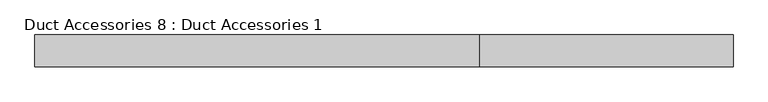
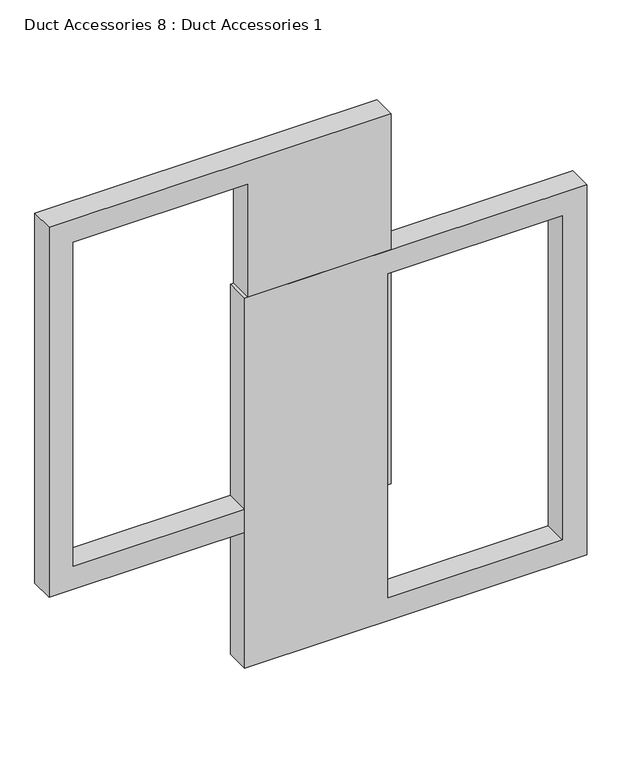
"""IFC4 building model written with IfcOpenShell, lengths in millimetres: damper geometry, Duct Accessories 8 : Duct Accessories 1."""

from ifc_helpers import new_model, si_unit, frame, origin, place, context, project, spatial, polyline, outline, extrude, source, transform, mapped, element, save


def duct_accessories_8_duct_accessories_1_4ac22e68(model_context):
    return source(origin(), model_context, "Body", "SweptSolid", [
        extrude(outline(polyline([(16734.3403114, -12928.36893), (15515.1403114, -12928.36893), (15515.1403114, -11861.56893), (16734.3403114, -11861.56893), (16734.3403114, -12928.36893)]), holes=[polyline([(16658.1403114, -12480.9324751), (16658.1403114, -11937.76893), (15591.3403114, -11937.76893), (15591.3403114, -12480.9324751), (16658.1403114, -12480.9324751)])]), frame((0.0, -447.4934478, 0.0), z_axis=(0.0, 1.0, 0.0), x_axis=(0.0, 0.0, 1.0)), (0.0, 0.0, 1.0), 76.2),
        extrude(outline(polyline([(17181.7767663, -12471.5606701), (17181.7767663, -13538.3606701), (15962.5767663, -13538.3606701), (15962.5767663, -12471.5606701), (17181.7767663, -12471.5606701)]), holes=[polyline([(17105.5767663, -12918.997125), (16038.7767663, -12918.997125), (16038.7767663, -13462.1606701), (17105.5767663, -13462.1606701), (17105.5767663, -12918.997125)])]), frame((0.0, -447.4934478, 0.0), z_axis=(0.0, 1.0, 0.0), x_axis=(0.0, 0.0, 1.0)), (0.0, 0.0, 1.0), 76.2),
    ])


if __name__ == "__main__":
    model = new_model("IFC4")
    model_context = context("Model", 3, world=origin())
    ifc_project = project(units=[si_unit("LENGTHUNIT", "METRE", prefix="MILLI")], contexts=[model_context])
    site = spatial("IfcSite", under=ifc_project)
    building = spatial("IfcBuilding", under=site)
    placement = place(None, origin())
    duct_accessories_8_duct_accessories_1_shape = duct_accessories_8_duct_accessories_1_4ac22e68(model_context)
    element("IfcDamper", 1, ObjectType="Duct Accessories 8 : Duct Accessories 1", at=placement, inside=building, context=model_context, shape_type="MappedRepresentation", body=[
        mapped(duct_accessories_8_duct_accessories_1_shape, transform((0.0, 0.0, 0.0), x_axis=(1.0, 0.0, 0.0), y_axis=(0.0, 1.0, 0.0), z_axis=(0.0, 0.0, 1.0))),
    ])
    save(model, "model.ifc")

# Revit data of these elements
# Element 1 (IfcDamper, "Duct Accessories 8 : Duct Accessories 1")
#   Materials on its faces: "border"
# Materials
#   "border": class "Generic", colour RGB 144 144 144, transparency 0, Cost = 0
